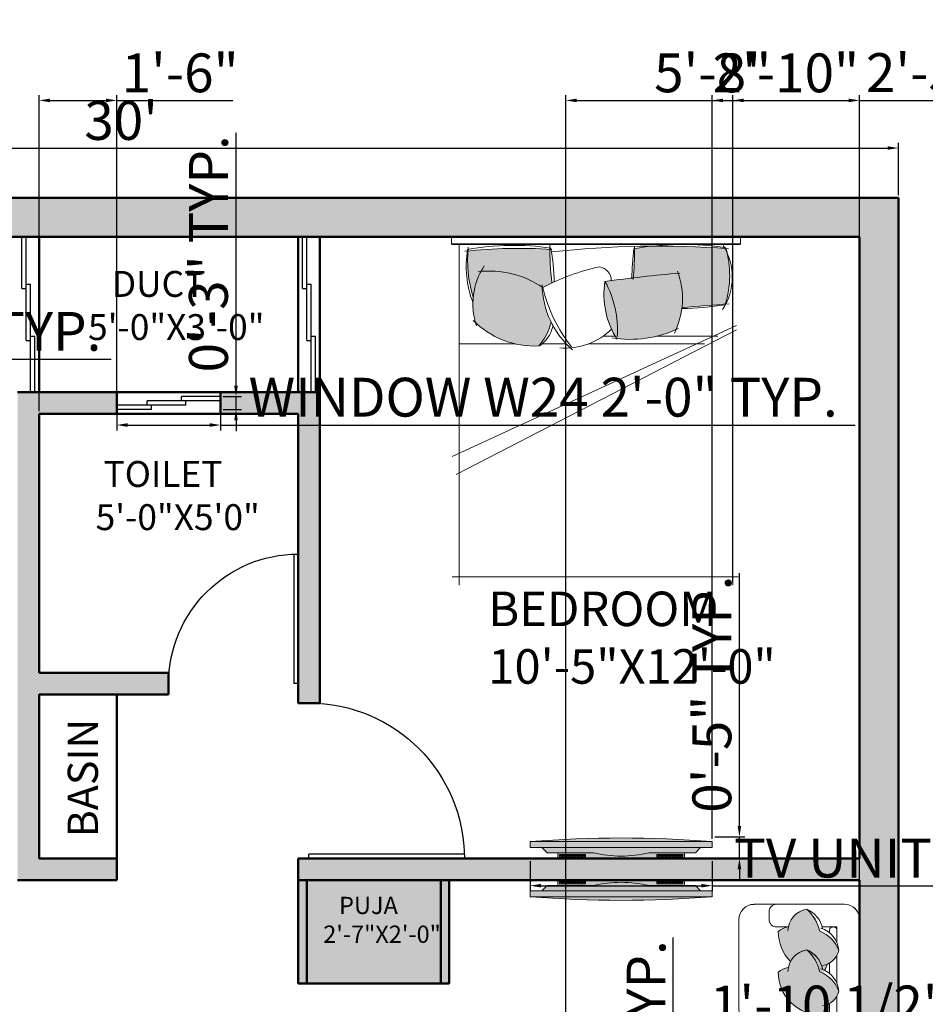
# Model space of a CAD drawing. Units: inches. Extents: x 3274 to 5176, y 1085 to 2172.
# Tile 8 of 16: x 3530 to 3740, y 1848 to 2076. Entities that reach past the tile are written whole.
import ezdxf

# ---------------------------------------------------------------- set-up
doc = ezdxf.new("R2010")
doc.units = ezdxf.units.IN
for name, color, linetype, lineweight in [('0.10', 252, 'Continuous', 9), ('A-ANNO-DIMS', 2, 'Continuous', 18), ('A-AREA-IDEN', 3, 'Continuous', 25), ('A-DOOR', 4, 'Continuous', 25), ('A-EQPM', 8, 'Continuous', 18), ('A-FLOR-PATT', 252, 'Continuous', 13), ('A-FURN', 8, 'Continuous', 18), ('A-GLAZ', 5, 'Continuous', 25), ('A-WALL', 7, 'Continuous', 50), ('A-WALL-PATT', 8, 'Continuous', 13), ('moveis', 254, 'Continuous', 5), ('parede', 7, 'Continuous', 30)]:
    doc.layers.add(name, color=color, linetype=linetype, lineweight=lineweight)
doc.styles.get("Standard").update_dxf_attribs({"font": 'arial.ttf'})
doc.dimstyles.new('ISO-25', dxfattribs={"dimtxt": 9, "dimasz": 2.5, "dimexe": 1.25, "dimexo": 0.625, "dimtad": 1, "dimdec": 1, "dimlunit": 3, "dimtxsty": 'Standard', "dimcen": 2.5, "dimclrd": 4, "dimclre": 4, "dimclrt": 1, "dimadec": 0, "dimazin": 0, "dimtfac": 1, "dimtdec": 1, "dimtmove": 0, "dimatfit": 3, "dimfxl": 1, "dimarcsym": 0})

# ---------------------------------------------------------------- blocks, each defined once
blk = doc.blocks.new('2')
for p, q in [((0, 30), (0, 0)), ((1, 30), (1, 0)), ((0, 0), (1, 0))]:
    blk.add_line(p, q)
blk.add_arc((0, 0), 30, 0, 90)
blk = doc.blocks.new('1')
for p, q in [((0, 36), (0, 0)), ((1, 36), (1, 0)), ((0, 0), (1, 0))]:
    blk.add_line(p, q)
blk.add_arc((0, 0), 36, 0, 90)
blk = doc.blocks.new('*D67')
at = {"layer": 'A-ANNO-DIMS', "color": 0, "lineweight": -2, "transparency": 16777216}
for p, q in [((3373.3, 2035.11), (3373.3, 2047.29)), ((3733.3, 2035.11), (3733.3, 2047.29)), ((3375.8, 2046.04), (3730.8, 2046.04))]:
    blk.add_line(p, q, dxfattribs=at)
at = {"layer": 'A-ANNO-DIMS', "color": 0, "transparency": 16777216}
for points in [[(3375.8, 2046.46), (3375.8, 2045.63), (3373.3, 2046.04)], [(3730.8, 2046.46), (3730.8, 2045.63), (3733.3, 2046.04)]]:
    blk.add_solid(points, dxfattribs=at)
at = {"layer": 'Defpoints', "color": 0, "transparency": 16777216}
for p in [(3733.3, 2046.04), (3373.3, 2034.48), (3733.3, 2034.48)]:
    blk.add_point(p, dxfattribs=at)
at = {"layer": 'A-ANNO-DIMS', "color": 0, "transparency": 16777216, "insert": (3553.3, 2051.27), "char_height": 9, "attachment_point": 5}
blk.add_mtext("30'", dxfattribs=at)
blk = doc.blocks.new('camita')
at = {"layer": '0.10'}
for p, q in [((-0.85, -0.045), (0.85, -0.045)), ((-0.805, -0.045), (-0.805, -2.0485)), ((0.805, -0.045), (0.805, -2.0485)), ((-0.8271, -0.521), (0.8464, -1.2932)), ((-0.8271, -0.5476), (0.8236, -1.3992)), ((-0.7161, -0.585), (-0.3554, -0.585)), ((-0.638, -0.63), (0.0434, -0.63)), ((-0.1136, -0.585), (-0.0485, -0.585)), ((0.1749, -0.63), (0.3179, -0.63)), ((0.4739, -0.63), (0.805, -0.63)), ((-0.8354, -2), (0.8464, -2))]:
    blk.add_line(p, q, dxfattribs=at)
blk.add_lwpolyline([(-0.85, -0.0405), (0.85, -0.0405), (0.85, 0), (-0.85, 0)], close=True, dxfattribs=at)
for centre, radius, start, end in [((-0.4574, -0.2364), 0.3443, 147.50996, 213.83359), ((-0.3639, -5.8457), 5.7909, 83.80731, 94.12107), ((-0.5104, -1.7232), 1.6781, 80.12554, 98.66187), ((-1.4396, -0.0609), 1.7117, 352.92911, 0.39592), ((0.4863, -1.6286), 1.5781, 80.16015, 98.05996), ((-0.1997, -0.2266), 0.5864, 163.92635, 197.14087), ((2.3534, -0.0532), 2.5803, 180.10628, 184.38541), ((-1.5443, -0.2452), 1.3333, 359.93941, 7.55329), ((1.5815, -0.2893), 1.3353, 170.38021, 178.99138), ((0.4524, -3.0675), 2.9996, 83.90257, 93.67595), ((0.0294, -0.1377), 0.7262, 342.58415, 6.00484), ((0.1326, -0.1696), 0.6307, 339.92303, 8.74334), ((0.3203, -0.3944), 0.4043, 341.45245, 33.45121), ((-0.0543, -0.3633), 0.4542, 159.30257, 206.50263), ((-1.3301, -9.6748), 9.4985, 82.27078, 84.93989), ((-0.007, -0.258), 0.0828, 100.01798, 179.73597), ((-0.2931, -1.4378), 1.2903, 61.97485, 77.84351), ((0.6265, -0.7518), 0.5508, 82.96906, 124.67388), ((0.4585, -0.5454), 0.5842, 151.04555, 184.14969), ((-0.5341, -0.3393), 0.4875, 327.26442, 9.0473), ((-0.1986, -0.2742), 0.5159, 310.73945, 359.05759), ((-0.5673, -0.0868), 0.9057, 321.69527, 346.46261), ((-1.8672, -14.986), 14.6323, 84.65974, 85.75157), ((-0.4598, 1.4861), 1.9092, 260.95299, 268.65169), ((0.5707, -0.4317), 0.3145, 192.93877, 221.96363), ((0.3612, -0.133), 0.5096, 267.25889, 315.29965), ((-0.2002, 0.064), 0.6673, 244.78094, 279.06058), ((0.179, -0.272), 0.3828, 224.52836, 275.22287), ((0.4384, -0.4834), 0.1898, 193.68485, 236.70352)]:
    blk.add_arc(centre, radius, start, end, dxfattribs=at)
blk = doc.blocks.new('SOFA 1')
at = {"transparency": 33554687}
h = blk.add_hatch(color=256, dxfattribs=at)
h.dxf.hatch_style = 1
h.paths.add_polyline_path([(3723.52, 1308.63, 0.147724), (3717.76, 1305.24, 0.310469), (3722.42, 1300.4), (3722.42, 1300.25, 0.156703), (3723.62, 1297.8, 0.425821), (3734.69, 1309.08, 0.121928), (3732.05, 1310.63, 0.233216), (3728.6, 1313.59, 0.213835)])
h = blk.add_hatch(color=256, dxfattribs=at)
h.dxf.hatch_style = 1
h.paths.add_polyline_path([(3769.65, 1307.6, 0.084911), (3767.15, 1309.12, 0.046133), (3766.46, 1311.13), (3759.18, 1311.13, 0.039409), (3758.92, 1310.24, 0.165523), (3756.31, 1309.02, 0.42585), (3767.59, 1297.95, 0.121928), (3769.15, 1300.58, 0.027403), (3769.65, 1300.83)])
h.paths.add_polyline_path([(3765.34, 1313.08), (3760.4, 1313.08, 0.097704), (3759.18, 1311.13), (3766.46, 1311.13, 0.04873)])
h.paths.add_polyline_path([(3763.76, 1314.88, 0.16488), (3760.4, 1313.08), (3765.34, 1313.08, 0.051917)])
h.paths.add_polyline_path([(3771.6, 1305.17, 0.090388), (3769.65, 1307.6), (3769.65, 1300.83, 0.136035), (3771.6, 1302.77)])
h = blk.add_hatch(color=256, dxfattribs=at)
h.dxf.hatch_style = 1
h.paths.add_polyline_path([(3769.16, 1235.96, 0.122267), (3767.6, 1238.61, 0.425972), (3756.32, 1227.54, 0.165563), (3758.93, 1226.32, 0.309481), (3763.76, 1221.69, 0.002677), (3763.83, 1221.72, 0.146094), (3767.16, 1227.43, 0.212433), (3772.1, 1232.48, 0.235342)])
h = blk.add_hatch(color=256, dxfattribs=at)
h.dxf.hatch_style = 1
h.paths.add_polyline_path([(3769.16, 1225.36, 0.122267), (3767.6, 1228.01, 0.425972), (3756.32, 1216.94, 0.165563), (3758.93, 1215.72, 0.309481), (3763.76, 1211.09, 0.002677), (3763.83, 1211.12, 0.146094), (3767.16, 1216.83, 0.212433), (3772.1, 1221.88, 0.235342)])
for p, q in [((3720.45, 1316.13), (3773.58, 1316.13)), ((3777.51, 1312.19), (3777.51, 1213.72))]:
    blk.add_line(p, q, dxfattribs=at)
for points in [[(3717.76, 1305.24, -0.147724), (3723.52, 1308.63, -0.213355), (3728.59, 1313.59, 0.213355), (3723.52, 1308.63, 0.147724), (3717.76, 1305.24, -0.249545), (3722.86, 1309.34, 0.249545), (3717.75, 1305.25, 0.356779), (3723.4, 1300.28, -0.356779), (3717.76, 1305.24)], [(3728.58, 1313.6, -0.306333), (3732.42, 1309.31, 0.306333), (3728.58, 1313.6, 0.306674), (3722.72, 1308.89, -0.306674), (3728.58, 1313.6)], [(3763.76, 1314.88, -0.147724), (3767.15, 1309.12, -0.213355), (3772.1, 1304.05, 0.213355), (3767.15, 1309.12, 0.147724), (3763.76, 1314.88, -0.249545), (3767.86, 1309.77, 0.249545), (3763.77, 1314.89, 0.356779), (3758.8, 1309.23, -0.356779), (3763.76, 1314.88)], [(3734.69, 1309.08, -0.425972), (3723.62, 1297.8, -0.165552), (3722.4, 1300.4, 0.165552), (3723.62, 1297.79, 0.425972), (3734.69, 1309.07, 0.121514), (3732.07, 1310.63, -0.121514), (3734.69, 1309.08)], [(3767.6, 1297.95, -0.425972), (3756.31, 1309.01, -0.165552), (3758.92, 1310.24, 0.165552), (3756.31, 1309.02, 0.425972), (3767.59, 1297.95, 0.121514), (3769.14, 1300.57, -0.121514), (3767.6, 1297.95)], [(3772.11, 1304.06, -0.306333), (3767.83, 1300.22, 0.306333), (3772.11, 1304.06, 0.306674), (3767.4, 1309.91, -0.306674), (3772.11, 1304.06)], [(3770.44, 1286.63, -0.414214), (3769.66, 1287.4, 0.414214), (3770.44, 1286.63, 0.414214), (3769.66, 1285.83, -0.414214), (3770.44, 1286.63)], [(3748.01, 1262.99, -0.414214), (3746.05, 1264.95, 0.414214), (3748.01, 1262.97, 0.414213), (3746.05, 1261.01, -0.414213), (3748.01, 1262.99)], [(3770.44, 1262.99, -0.414214), (3769.66, 1263.77, 0.414214), (3770.44, 1262.99, 0.414214), (3769.66, 1262.19, -0.414214), (3770.44, 1262.99)], [(3770.83, 1262.97, -0.414214), (3771.61, 1262.19, 0.414214), (3770.83, 1262.99, 0.414214), (3771.61, 1263.77, -0.414214), (3770.83, 1262.97)], [(3748.01, 1239.35, -0.414214), (3746.05, 1241.31, 0.414214), (3748.01, 1239.33, 0.414213), (3746.05, 1237.37, -0.414213), (3748.01, 1239.35)], [(3767.7, 1239.33, -0.414214), (3769.66, 1237.37, 0.414214), (3767.7, 1239.35, 0.414214), (3769.66, 1241.31, -0.414214), (3767.7, 1239.33)], [(3756.32, 1227.54, -0.425972), (3767.6, 1238.61, -0.121514), (3769.16, 1235.98, 0.121514), (3767.6, 1238.61, 0.425972), (3756.32, 1227.54, 0.165552), (3758.93, 1226.32, -0.165552), (3756.32, 1227.54)], [(3770.44, 1239.35, -0.414214), (3769.66, 1240.13, 0.414214), (3770.44, 1239.33, 0.414214), (3769.66, 1238.55, -0.414214), (3770.44, 1239.35)], [(3770.83, 1239.33, -0.414214), (3771.61, 1238.55, 0.414214), (3770.83, 1239.35, 0.414214), (3771.61, 1240.13, -0.414214), (3770.83, 1239.33)], [(3772.1, 1232.5, -0.306674), (3767.41, 1226.64, 0.306674), (3772.1, 1232.5, 0.306333), (3767.84, 1236.34, -0.306333), (3772.1, 1232.5)], [(3763.78, 1221.67, 0.249545), (3767.87, 1226.78, -0.249545), (3763.76, 1221.69, -0.356779), (3758.81, 1227.32, 0.356779), (3763.77, 1221.68, 0.147724), (3767.16, 1227.43, 0.213355), (3772.11, 1232.51, -0.213355), (3767.16, 1227.43, -0.147724), (3763.78, 1221.67)], [(3756.32, 1216.94, -0.200233), (3759.49, 1224.76, 0.200233), (3756.32, 1216.94, 0.165552), (3758.93, 1215.72, -0.165552), (3756.32, 1216.94)], [(3772.1, 1221.9, -0.306674), (3767.41, 1216.04, 0.306674), (3772.1, 1221.9, -0.213355), (3767.16, 1216.83, -0.147724), (3763.77, 1211.08, 0.147724), (3767.15, 1216.83, 0.213355), (3772.1, 1221.9)], [(3763.76, 1211.09, -0.356779), (3758.81, 1216.72, 0.356779), (3763.76, 1211.09, 0.249545), (3767.87, 1216.18, -0.249545), (3763.76, 1211.09)]]:
    blk.add_lwpolyline(points, format="xyb", dxfattribs=at)
for points in [[(3716.51, 1312.2), (3716.51, 1291.44)], [(3722.42, 1313.08), (3722.42, 1309.23), (3722.42, 1313.08), (3726.57, 1313.08)], [(3723.21, 1311.13), (3723.93, 1311.13)], [(3729.85, 1313.08), (3745.25, 1313.08)], [(3731.82, 1311.13), (3745.25, 1311.13)], [(3746.01, 1312.3), (3746.01, 1288.55)], [(3746.01, 1310.97), (3746.01, 1311.36)], [(3768.11, 1313.08), (3746.78, 1313.08)], [(3768.87, 1311.13), (3746.78, 1311.13)], [(3771.6, 1313.08), (3767.75, 1313.08), (3771.6, 1313.08), (3771.6, 1308.93)], [(3769.66, 1287.39), (3769.65, 1312.3)], [(3771.6, 1313.08), (3771.61, 1233.74)], [(3746.01, 1288.54), (3746.01, 1308.23)], [(3769.65, 1309.43), (3769.65, 1308.71)], [(3722.42, 1300.39), (3722.42, 1297.33)], [(3720.45, 1295.38), (3718.48, 1295.38)], [(3720.45, 1287.5), (3744.09, 1287.5)], [(3747.99, 1286.6), (3767.69, 1286.6)], [(3769.66, 1263.75), (3769.66, 1285.81)], [(3746.02, 1284.63), (3746.02, 1264.94)], [(3769.66, 1277.18), (3769.66, 1263.75)], [(3747.99, 1262.97), (3767.69, 1262.97)], [(3769.66, 1240.12), (3769.66, 1262.18)], [(3770.43, 1262.97), (3770.82, 1262.97)], [(3746.02, 1260.99), (3746.02, 1241.3)], [(3747.99, 1239.33), (3767.69, 1239.33)], [(3770.43, 1239.33), (3770.82, 1239.33)], [(3746.02, 1237.36), (3746.02, 1213.74)], [(3769.66, 1235.71), (3769.66, 1238.54)], [(3771.61, 1223.14), (3771.61, 1230.47)], [(3769.66, 1225.11), (3769.66, 1227.82)], [(3767.76, 1215.72), (3771.61, 1215.72), (3771.61, 1219.84), (3771.61, 1215.72)], [(3755.86, 1215.72), (3758.92, 1215.72)], [(3769.66, 1216.5), (3769.66, 1217.22)], [(3753.91, 1211.77), (3753.91, 1213.74)], [(3749.97, 1209.8), (3773.58, 1209.8)]]:
    blk.add_lwpolyline(points, close=True, dxfattribs=at)
for points in [[(3722.42, 1311.91, 0.414214), (3723.2, 1311.13, -0.414214)], [(3770.43, 1313.08, 0.414214), (3769.65, 1312.3, -0.414214)], [(3771.6, 1312.3, 0.414214), (3770.82, 1313.08, -0.414214)], [(3716.51, 1297.34, 0.414214), (3718.47, 1295.38, -0.414214)], [(3720.44, 1295.38, 0.414214), (3722.4, 1297.34, -0.414214)], [(3716.51, 1291.45, 0.414212), (3720.44, 1287.52, -0.414212)], [(3746.03, 1288.56, 0.414214), (3747.99, 1286.6, 0.414213), (3746.03, 1284.64, -0.414213), (3747.99, 1286.6, -0.414214)], [(3769.66, 1284.64, 0.414214), (3767.7, 1286.6, 0.414214), (3769.66, 1288.56, -0.414214), (3767.7, 1286.6, -0.414214)], [(3769.66, 1261.01, 0.414214), (3767.7, 1262.97, 0.414214), (3769.66, 1264.93, -0.414214), (3767.7, 1262.97, -0.414214)], [(3769.16, 1225.36, 0.071861), (3768.39, 1227.01, -0.071861)], [(3772.13, 1221.9, 0.306333), (3767.84, 1225.74, -0.306333)], [(3755.87, 1215.72, 0.414214), (3753.91, 1213.76, -0.414214)], [(3769.66, 1216.52, 0.414214), (3770.44, 1215.74, -0.414214)], [(3770.83, 1215.74, 0.414214), (3771.61, 1216.52, -0.414214)], [(3746.05, 1213.76, 0.414212), (3749.98, 1209.82, -0.414212)], [(3755.87, 1209.8, -0.414214), (3753.91, 1211.76, 0.414214)]]:
    blk.add_lwpolyline(points, format="xyb", close=True, dxfattribs=at)
for centre, radius, start, end in [((3720.44, 1312.2), 3.93, 90.0002, 179.9998), ((3720.44, 1312.19), 3.94, 89.9158, 179.9154), ((3773.58, 1312.2), 3.93, 0.0002, 89.9998), ((3773.57, 1312.19), 3.94, 359.9158, 89.9154), ((3744.09, 1309.21), 1.92, 358.766, 90.5111), ((3745.22, 1312.29), 0.789, 0.8425, 90.8425), ((3745.24, 1311.91), 0.777, 270, 0), ((3745.24, 1311.91), 0.777, 270, 0), ((3746.8, 1312.29), 0.789, 89.1575, 179.1575), ((3746.79, 1311.91), 0.777, 180, 270), ((3746.79, 1311.91), 0.777, 180, 270), ((3747.93, 1309.21), 1.92, 89.4889, 181.234), ((3768.87, 1312.3), 0.777, 360, 90), ((3768.87, 1311.91), 0.777, 270, 0), ((3744.08, 1289.48), 1.96, 270, 360), ((3744.08, 1289.48), 1.96, 270, 360), ((3773.58, 1213.73), 3.93, 270.0002, 359.9998), ((3773.59, 1213.73), 3.93, 269.9156, 359.9152)]:
    blk.add_arc(centre, radius, start, end, dxfattribs=at)
blk = doc.blocks.new('PLASMA 2')
at = {"layer": 'moveis', "ltscale": 0.08}
h = blk.add_hatch(dxfattribs=at)
h.set_pattern_fill('_USER,_O', color=256, scale=0.008, double=1, pattern_type=0)
h.set_pattern_definition([(360, (-4.134502, -6.848382), (0, 0.008), []), (90, (-4.134502, -6.848382), (-0.008, 0), [])])
h.paths.add_polyline_path([(-0.2099, -0.0965), (-0.3623, -0.0965), (-0.3623, -0.1111), (-0.2099, -0.1111)])
h = blk.add_hatch(dxfattribs=at)
h.set_pattern_fill('_USER,_O', color=256, scale=0.008, double=1, pattern_type=0)
h.set_pattern_definition([(180, (4.134502, -6.848382), (0, 0.008), []), (90, (4.134502, -6.848382), (0.008, 0), [])])
h.paths.add_polyline_path([(0.2099, -0.0965), (0.3623, -0.0965), (0.3623, -0.1111), (0.2099, -0.1111)])
at = {"layer": 'parede', "ltscale": 0.08}
h = blk.add_hatch(color=256, dxfattribs=at)
h.dxf.hatch_style = 1
h.set_gradient(color1=(131, 136, 145), one_color=1, tint=1, name='CURVED')
h.paths.add_polyline_path([(-0.535, -0.0215), (0.535, -0.0215, 0.040195)])
h = blk.add_hatch(color=256, dxfattribs=at)
h.dxf.hatch_style = 1
h.set_gradient(color1=(131, 136, 145), color2=(0, 0, 0), one_color=1, name='CURVED')
h.paths.add_polyline_path([(0.535, -0.0215), (-0.535, -0.0215), (-0.535, -0.0553), (0.535, -0.0553)])
h = blk.add_hatch(color=256, dxfattribs=at)
h.dxf.hatch_style = 1
h.set_gradient(color1=(131, 136, 145), one_color=1, tint=1, name='CYLINDER')
h.paths.add_polyline_path([(0.4673, -0.0553), (-0.4673, -0.0553), (-0.4363, -0.0876), (-0.1636, -0.0876, 0.114423), (0.1636, -0.0876), (0.4363, -0.0876)])
h = blk.add_hatch(color=256, dxfattribs=at)
h.dxf.hatch_style = 1
h.set_gradient(color1=(131, 136, 145), color2=(0, 0, 0), one_color=1, name='CURVED')
h.paths.add_polyline_path([(0.3724, -0.0876), (0.1636, -0.0876, -0.114423), (-0.1636, -0.0876), (-0.3724, -0.0876), (-0.3724, -0.12), (0.3724, -0.12)])
h.paths.add_polyline_path([(-0.2099, -0.1111), (-0.3623, -0.1111), (-0.3623, -0.0965), (-0.2099, -0.0965)], flags=16)
h.paths.add_polyline_path([(0.2099, -0.1111), (0.2099, -0.0965), (0.3623, -0.0965), (0.3623, -0.1111)], flags=16)
at = {"layer": 'moveis', "ltscale": 0.08}
for p, q in [((-0.535, -0.0215), (-0.535, -0.0553)), ((-0.535, -0.0215), (0.535, -0.0215)), ((0.535, -0.0553), (-0.535, -0.0553)), ((-0.4673, -0.0553), (-0.4363, -0.0876)), ((0.4673, -0.0553), (0.4363, -0.0876)), ((0.535, -0.0553), (0.535, -0.0215)), ((-0.4363, -0.0876), (-0.1636, -0.0876)), ((-0.3724, -0.0876), (-0.3724, -0.12)), ((0.1636, -0.0876), (0.4363, -0.0876)), ((0.3724, -0.0876), (0.3724, -0.12)), ((-0.3724, -0.12), (0.3724, -0.12))]:
    blk.add_line(p, q, dxfattribs=at)
for points in [[(-0.3623, -0.0965), (-0.2099, -0.0965), (-0.2099, -0.1111), (-0.3623, -0.1111)], [(0.3623, -0.0965), (0.2099, -0.0965), (0.2099, -0.1111), (0.3623, -0.1111)]]:
    blk.add_lwpolyline(points, close=True, dxfattribs=at)
for centre, radius, start, end in [((0, -6.6658), 6.6658, 85.39647, 94.60353), ((0, 0.6178), 0.7242, 256.94486, 283.05514)]:
    blk.add_arc(centre, radius, start, end, dxfattribs=at)
blk = doc.blocks.new('WIN-24')
for p, q in [((4551.19, 1486.35), (4551.19, 1487.35)), ((4560.19, 1487.35), (4551.19, 1487.35)), ((4552.19, 1485.35), (4536.19, 1485.35)), ((4560.19, 1486.35), (4543.19, 1486.35)), ((4543.19, 1485.35), (4543.19, 1486.35)), ((4544.19, 1484.35), (4544.19, 1485.35)), ((4552.19, 1485.35), (4552.19, 1486.35)), ((4544.19, 1484.35), (4536.19, 1484.35))]:
    blk.add_line(p, q)
blk = doc.blocks.new('WIN-36')
for p, q in [((4514.19, 1512.35), (4514.19, 1524.35)), ((4515.19, 1500.35), (4515.19, 1524.35)), ((4514.19, 1512.35), (4515.19, 1512.35)), ((4515.19, 1513.35), (4516.19, 1513.35)), ((4516.19, 1488.35), (4516.19, 1513.35)), ((4516.19, 1501.35), (4517.19, 1501.35)), ((4517.19, 1488.35), (4517.19, 1501.35)), ((4515.19, 1500.35), (4516.19, 1500.35))]:
    blk.add_line(p, q)
blk = doc.blocks.new('*D126')
at = {"layer": 'A-ANNO-DIMS', "color": 4, "lineweight": -2, "transparency": 16777216}
for p, q in [((3552.3, 1984.86), (3552.3, 1980.63)), ((3576.3, 1984.86), (3576.3, 1980.63)), ((3554.8, 1981.88), (3573.8, 1981.88)), ((3576.3, 1981.88), (3723.28, 1981.88))]:
    blk.add_line(p, q, dxfattribs=at)
at = {"layer": 'A-ANNO-DIMS', "color": 4, "transparency": 16777216}
for points in [[(3554.8, 1982.3), (3554.8, 1981.47), (3552.3, 1981.88)], [(3573.8, 1982.3), (3573.8, 1981.47), (3576.3, 1981.88)]]:
    blk.add_solid(points, dxfattribs=at)
at = {"layer": 'Defpoints', "color": 0, "transparency": 16777216}
for p in [(3552.3, 1985.48), (3576.3, 1985.48), (3576.3, 1981.88)]:
    blk.add_point(p, dxfattribs=at)
at = {"layer": 'A-ANNO-DIMS', "color": 1, "transparency": 16777216, "insert": (3651.04, 1987.16), "char_height": 9, "attachment_point": 5}
blk.add_mtext('WINDOW W24 2\'-0" TYP.', dxfattribs=at)
blk = doc.blocks.new('*D127')
at = {"layer": 'A-ANNO-DIMS', "color": 4, "lineweight": -2, "transparency": 16777216}
for p, q in [((3579.9, 1990.98), (3579.9, 2049.59)), ((3576.93, 1988.48), (3581.15, 1988.48)), ((3579.9, 1985.48), (3579.9, 1988.48)), ((3576.93, 1985.48), (3581.15, 1985.48)), ((3579.9, 1982.98), (3579.9, 1980.48))]:
    blk.add_line(p, q, dxfattribs=at)
at = {"layer": 'A-ANNO-DIMS', "color": 4, "transparency": 16777216}
for points in [[(3579.48, 1990.98), (3580.32, 1990.98), (3579.9, 1988.48)], [(3579.48, 1982.98), (3580.32, 1982.98), (3579.9, 1985.48)]]:
    blk.add_solid(points, dxfattribs=at)
at = {"layer": 'Defpoints', "color": 0, "transparency": 16777216}
for p in [(3576.3, 1988.48), (3579.9, 1988.48), (3576.3, 1985.48)]:
    blk.add_point(p, dxfattribs=at)
at = {"layer": 'A-ANNO-DIMS', "color": 1, "transparency": 16777216, "insert": (3574.68, 2021.54), "char_height": 9, "attachment_point": 5, "rotation": 90}
blk.add_mtext('0\'-3" TYP.', dxfattribs=at)
blk = doc.blocks.new('*D130')
at = {"layer": 'A-ANNO-DIMS', "color": 4, "lineweight": -2, "transparency": 16777216}
for p, q in [((3648.04, 1880.86), (3648.04, 1873.91)), ((3690.17, 1880.86), (3690.17, 1873.91)), ((3650.54, 1875.16), (3687.67, 1875.16)), ((3690.17, 1875.16), (3801.39, 1875.16))]:
    blk.add_line(p, q, dxfattribs=at)
at = {"layer": 'A-ANNO-DIMS', "color": 4, "transparency": 16777216}
for points in [[(3650.54, 1875.58), (3650.54, 1874.75), (3648.04, 1875.16)], [(3687.67, 1875.58), (3687.67, 1874.75), (3690.17, 1875.16)]]:
    blk.add_solid(points, dxfattribs=at)
at = {"layer": 'Defpoints', "color": 0, "transparency": 16777216}
for p in [(3648.04, 1881.48), (3690.17, 1881.48), (3690.17, 1875.16)]:
    blk.add_point(p, dxfattribs=at)
at = {"layer": 'A-ANNO-DIMS', "color": 1, "transparency": 16777216, "insert": (3747.03, 1880.39), "char_height": 9, "attachment_point": 5}
blk.add_mtext('TV UNIT 3\'-6" TYP.', dxfattribs=at)
blk = doc.blocks.new('*D131')
at = {"layer": 'A-ANNO-DIMS', "color": 4, "lineweight": -2, "transparency": 16777216}
for p, q in [((3696.49, 1888.99), (3696.49, 1947.6)), ((3690.79, 1886.49), (3697.74, 1886.49)), ((3696.49, 1881.48), (3696.49, 1886.49)), ((3690.79, 1881.48), (3697.74, 1881.48)), ((3696.49, 1878.98), (3696.49, 1876.48))]:
    blk.add_line(p, q, dxfattribs=at)
at = {"layer": 'A-ANNO-DIMS', "color": 4, "transparency": 16777216}
for points in [[(3696.07, 1888.99), (3696.9, 1888.99), (3696.49, 1886.49)], [(3696.07, 1878.98), (3696.9, 1878.98), (3696.49, 1881.48)]]:
    blk.add_solid(points, dxfattribs=at)
at = {"layer": 'Defpoints', "color": 0, "transparency": 16777216}
for p in [(3690.17, 1886.49), (3696.49, 1886.49), (3690.17, 1881.48)]:
    blk.add_point(p, dxfattribs=at)
at = {"layer": 'A-ANNO-DIMS', "color": 1, "transparency": 16777216, "insert": (3691.27, 1919.54), "char_height": 9, "attachment_point": 5, "rotation": 90}
blk.add_mtext('0\'-5" TYP.', dxfattribs=at)
blk = doc.blocks.new('*D139')
at = {"layer": 'A-ANNO-DIMS', "color": 4, "lineweight": -2, "transparency": 16777216}
for p, q in [((3664.71, 1838.01), (3664.71, 1842.31)), ((3667.21, 1841.06), (3684.52, 1841.06)), ((3687.02, 1838.01), (3687.02, 1842.31)), ((3687.02, 1841.06), (3772.75, 1841.06))]:
    blk.add_line(p, q, dxfattribs=at)
at = {"layer": 'A-ANNO-DIMS', "color": 4, "transparency": 16777216}
for points in [[(3667.21, 1841.48), (3667.21, 1840.65), (3664.71, 1841.06)], [(3684.52, 1841.48), (3684.52, 1840.65), (3687.02, 1841.06)]]:
    blk.add_solid(points, dxfattribs=at)
at = {"layer": 'Defpoints', "color": 0, "transparency": 16777216}
for p in [(3687.02, 1841.06), (3664.71, 1837.38), (3687.02, 1837.38)]:
    blk.add_point(p, dxfattribs=at)
at = {"layer": 'A-ANNO-DIMS', "color": 1, "transparency": 16777216, "insert": (3731.13, 1846.34), "char_height": 9, "attachment_point": 5}
blk.add_mtext('1\'-10 1/2" TYP.', dxfattribs=at)
blk = doc.blocks.new('*D141')
at = {"layer": 'A-ANNO-DIMS', "color": 4, "lineweight": -2, "transparency": 16777216}
for p, q in [((3681.18, 1804.42), (3681.18, 1863.19)), ((3670.79, 1804.42), (3682.43, 1804.42)), ((3681.18, 1778.97), (3681.18, 1801.92)), ((3670.79, 1776.47), (3682.43, 1776.47))]:
    blk.add_line(p, q, dxfattribs=at)
at = {"layer": 'A-ANNO-DIMS', "color": 4, "transparency": 16777216}
for points in [[(3680.76, 1801.92), (3681.59, 1801.92), (3681.18, 1804.42)], [(3680.76, 1778.97), (3681.59, 1778.97), (3681.18, 1776.47)]]:
    blk.add_solid(points, dxfattribs=at)
at = {"layer": 'Defpoints', "color": 0, "transparency": 16777216}
for p in [(3670.16, 1804.42), (3681.18, 1804.42), (3670.16, 1776.47)]:
    blk.add_point(p, dxfattribs=at)
at = {"layer": 'A-ANNO-DIMS', "color": 1, "transparency": 16777216, "insert": (3676.03, 1835.06), "char_height": 9, "attachment_point": 5, "rotation": 90}
blk.add_mtext('2\'-4" TYP.', dxfattribs=at)
blk = doc.blocks.new('*D144')
at = {"layer": 'A-ANNO-DIMS', "color": 4, "lineweight": -2, "transparency": 16777216}
for p, q in [((3382.3, 2005.96), (3382.3, 1995.89)), ((3445.29, 2005.96), (3445.29, 1995.89)), ((3384.8, 1997.14), (3442.79, 1997.14)), ((3445.29, 1997.14), (3551.01, 1997.14))]:
    blk.add_line(p, q, dxfattribs=at)
at = {"layer": 'A-ANNO-DIMS', "color": 4, "transparency": 16777216}
for points in [[(3384.8, 1997.55), (3384.8, 1996.72), (3382.3, 1997.14)], [(3442.79, 1997.55), (3442.79, 1996.72), (3445.29, 1997.14)]]:
    blk.add_solid(points, dxfattribs=at)
at = {"layer": 'Defpoints', "color": 0, "transparency": 16777216}
for p in [(3382.3, 2006.59), (3445.29, 2006.59), (3445.29, 1997.14)]:
    blk.add_point(p, dxfattribs=at)
at = {"layer": 'A-ANNO-DIMS', "color": 1, "transparency": 16777216, "insert": (3499.4, 2002.42), "char_height": 9, "attachment_point": 5}
blk.add_mtext('BENCH 5\'-3" TYP.', dxfattribs=at)
blk = doc.blocks.new('*D174')
at = {"layer": 'A-ANNO-DIMS', "color": 4, "lineweight": -2, "transparency": 16777216}
for p, q in [((3656.3, 1777.11), (3656.3, 2058.33)), ((3724.3, 1777.11), (3724.3, 2058.33)), ((3658.8, 2057.08), (3721.8, 2057.08))]:
    blk.add_line(p, q, dxfattribs=at)
at = {"layer": 'A-ANNO-DIMS', "color": 4, "transparency": 16777216}
for points in [[(3658.8, 2057.5), (3658.8, 2056.67), (3656.3, 2057.08)], [(3721.8, 2057.5), (3721.8, 2056.67), (3724.3, 2057.08)]]:
    blk.add_solid(points, dxfattribs=at)
at = {"layer": 'Defpoints', "color": 0, "transparency": 16777216}
for p in [(3724.3, 2057.08), (3656.3, 1776.48), (3724.3, 1776.48)]:
    blk.add_point(p, dxfattribs=at)
at = {"layer": 'A-ANNO-DIMS', "color": 1, "transparency": 16777216, "insert": (3690.3, 2062.3), "char_height": 9, "attachment_point": 5}
blk.add_mtext('5\'-8"', dxfattribs=at)
blk = doc.blocks.new('*D175')
at = {"layer": 'A-ANNO-DIMS', "color": 4, "lineweight": -2, "transparency": 16777216}
for p, q in [((3534.3, 1985.11), (3534.3, 2058.33)), ((3552.3, 1985.11), (3552.3, 2058.33)), ((3536.8, 2057.08), (3549.8, 2057.08)), ((3552.3, 2057.08), (3579.13, 2057.08))]:
    blk.add_line(p, q, dxfattribs=at)
at = {"layer": 'A-ANNO-DIMS', "color": 4, "transparency": 16777216}
for points in [[(3536.8, 2057.5), (3536.8, 2056.67), (3534.3, 2057.08)], [(3549.8, 2057.5), (3549.8, 2056.67), (3552.3, 2057.08)]]:
    blk.add_solid(points, dxfattribs=at)
at = {"layer": 'Defpoints', "color": 0, "transparency": 16777216}
for p in [(3552.3, 2057.08), (3534.3, 1984.48), (3552.3, 1984.48)]:
    blk.add_point(p, dxfattribs=at)
at = {"layer": 'A-ANNO-DIMS', "color": 1, "transparency": 16777216, "insert": (3566.96, 2062.3), "char_height": 9, "attachment_point": 5}
blk.add_mtext('1\'-6"', dxfattribs=at)
blk = doc.blocks.new('*D177')
at = {"layer": 'A-ANNO-DIMS', "color": 4, "lineweight": -2, "transparency": 16777216}
for p, q in [((3694.98, 1945.45), (3694.98, 2058.33)), ((3724.3, 1882.11), (3724.3, 2058.33)), ((3697.48, 2057.08), (3721.8, 2057.08)), ((3724.3, 2057.08), (3773.1, 2057.08))]:
    blk.add_line(p, q, dxfattribs=at)
at = {"layer": 'A-ANNO-DIMS', "color": 4, "transparency": 16777216}
for points in [[(3697.48, 2057.5), (3697.48, 2056.67), (3694.98, 2057.08)], [(3721.8, 2057.5), (3721.8, 2056.67), (3724.3, 2057.08)]]:
    blk.add_solid(points, dxfattribs=at)
at = {"layer": 'Defpoints', "color": 0, "transparency": 16777216}
for p in [(3724.3, 2057.08), (3694.98, 1944.83), (3724.3, 1881.48)]:
    blk.add_point(p, dxfattribs=at)
at = {"layer": 'A-ANNO-DIMS', "color": 1, "transparency": 16777216, "insert": (3749.95, 2062.36), "char_height": 9, "attachment_point": 5}
blk.add_mtext('2\'-5 1/2"', dxfattribs=at)
blk = doc.blocks.new('*D179')
at = {"layer": 'A-ANNO-DIMS', "color": 4, "lineweight": -2, "transparency": 16777216}
for p, q in [((3690.17, 1885.99), (3690.17, 2058.33)), ((3724.3, 1882.11), (3724.3, 2058.33)), ((3692.67, 2057.08), (3721.8, 2057.08))]:
    blk.add_line(p, q, dxfattribs=at)
at = {"layer": 'A-ANNO-DIMS', "color": 4, "transparency": 16777216}
for points in [[(3692.67, 2057.5), (3692.67, 2056.67), (3690.17, 2057.08)], [(3721.8, 2057.5), (3721.8, 2056.67), (3724.3, 2057.08)]]:
    blk.add_solid(points, dxfattribs=at)
at = {"layer": 'Defpoints', "color": 0, "transparency": 16777216}
for p in [(3724.3, 2057.08), (3690.17, 1885.36), (3724.3, 1881.48)]:
    blk.add_point(p, dxfattribs=at)
at = {"layer": 'A-ANNO-DIMS', "color": 1, "transparency": 16777216, "insert": (3707.24, 2062.3), "char_height": 9, "attachment_point": 5}
blk.add_mtext('2\'-10"', dxfattribs=at)

msp = doc.modelspace()

# ---------------------------------------------------------------- hatches: boundary and pattern name
at = {"layer": 'A-FLOR-PATT'}
h = msp.add_hatch(color=256, dxfattribs=at)
h.dxf.hatch_style = 1
h.paths.add_polyline_path([(3693.63, 2021.8, 0.020657), (3693.12, 2022.8, 0.01851), (3676.25, 2023.32, 0.015442), (3672.21, 2022.76, -0.016701), (3671.94, 2015.98, -0.006967), (3682.31, 2017.05, -0.113891), (3683.18, 2009.06, -0.004387), (3693.25, 2009.91, 0.131047)])
h.paths.add_polyline_path([(3682.31, 2017.05, 0.006967), (3671.94, 2015.98, 0.00444), (3665.35, 2015.14, 0.181694), (3668.06, 2001.91, 0.134508), (3681.79, 2003.97, 0.189536)])
h = msp.add_hatch(color=256, dxfattribs=at)
h.dxf.hatch_style = 1
h.paths.add_polyline_path([(3652.57, 2022.6, 0.040212), (3633.61, 2022.21, 0.094792), (3634.83, 2011.54, -0.098488), (3636.64, 2017.48, -0.175864), (3650.95, 2013.72, -0.011742), (3653.08, 2014.79, -0.029051)])
h.paths.add_polyline_path([(3650.81, 2013.81, 0.173835), (3636.64, 2017.48, 0.194952), (3635.36, 2005.59, 0.202559), (3650.02, 2000.2, 0.127326), (3652.88, 2005.71, -0.104045)])
h = msp.add_hatch(color=256, dxfattribs=at)
h.dxf.hatch_style = 1
h.paths.add_polyline_path([(3629.3, 1876.48), (3627.3, 1876.48), (3627.3, 1852.48), (3629.3, 1852.48)])
h.paths.add_polyline_path([(3596.3, 1876.48), (3594.3, 1876.48), (3594.3, 1852.48), (3596.3, 1852.48)])
h = msp.add_hatch(color=256, dxfattribs=at)
h.dxf.hatch_style = 1
h.paths.add_polyline_path([(3627.3, 1876.48), (3596.3, 1876.48), (3596.3, 1852.48), (3627.3, 1852.48)])
h.paths.add_polyline_path([(3598.94, 1859.73), (3626.92, 1859.73), (3626.92, 1874.65), (3598.94, 1874.65)], flags=24)
at = {"layer": 'A-WALL-PATT'}
h = msp.add_hatch(color=256, dxfattribs=at)
h.dxf.hatch_style = 1
h.paths.add_polyline_path([(3733.3, 2034.48), (3373.3, 2034.48), (3373.3, 1674.48), (3406.3, 1674.48), (3406.3, 1683.48), (3382.3, 1683.48), (3382.3, 1767.48), (3442.3, 1767.48), (3442.3, 1772.48), (3382.3, 1772.48), (3382.3, 1876.48), (3442.3, 1876.48), (3442.3, 1881.48), (3382.3, 1881.48), (3382.3, 2025.48), (3724.3, 2025.48), (3724.3, 1881.48), (3594.3, 1881.48), (3594.3, 1876.48), (3724.3, 1876.48), (3724.3, 1776.48), (3656.3, 1776.48), (3656.3, 1767.48), (3724.3, 1767.48), (3724.3, 1683.48), (3682.3, 1683.48), (3682.3, 1674.48), (3733.3, 1674.48)])
h.paths.add_polyline_path([(3477.3, 1876.48), (3493.3, 1876.48), (3493.3, 1881.48), (3472.3, 1881.48), (3472.3, 1820.48), (3417.3, 1820.48), (3417.3, 1840.48), (3412.3, 1840.48), (3412.3, 1815.48), (3472.3, 1815.48), (3472.3, 1767.48), (3493.3, 1767.48), (3493.3, 1772.48), (3477.3, 1772.48)], flags=17)
h.paths.add_polyline_path([(3534.3, 1984.48), (3552.3, 1984.48), (3552.3, 1989.48), (3529.3, 1989.48), (3529.3, 1876.48), (3552.3, 1876.48), (3552.3, 1881.48), (3534.3, 1881.48), (3534.3, 1919.48), (3564.3, 1919.48), (3564.3, 1924.48), (3534.3, 1924.48)], flags=17)
h.paths.add_polyline_path([(3599.3, 1989.48), (3576.3, 1989.48), (3576.3, 1984.48), (3594.3, 1984.48), (3594.3, 1917.48), (3599.3, 1917.48)], flags=17)
h.paths.add_polyline_path([(3534.3, 1767.48), (3539.3, 1767.48), (3539.3, 1776.48), (3529.3, 1776.48), (3529.3, 1683.48), (3478.3, 1683.48), (3478.3, 1674.48), (3534.3, 1674.48)], flags=17)
h.paths.add_polyline_path([(3596.3, 1776.48), (3587.3, 1776.48), (3587.3, 1771.98), (3587.3, 1767.48), (3596.3, 1767.48)], flags=17)
h.paths.add_polyline_path([(3610.3, 1683.48), (3594.3, 1683.48), (3594.3, 1674.48), (3610.3, 1674.48)], flags=17)
h.paths.add_polyline_path([(3589.35, 1817.42), (3663.55, 1817.42), (3663.55, 1847.27), (3589.35, 1847.27)], flags=25)
h.paths.add_polyline_path([(3545.54, 1954.13), (3584.72, 1954.13), (3584.72, 1976.52), (3545.54, 1976.52)], flags=25)
h.paths.add_polyline_path([(3635.11, 1944.89), (3703.51, 1944.89), (3703.51, 1974.74), (3635.11, 1974.74)], flags=25)
h.paths.add_polyline_path([(3543.78, 1998.17), (3585.75, 1998.17), (3585.75, 2020.56), (3543.78, 2020.56)], flags=25)
h.paths.add_polyline_path([(3423.19, 1944.89), (3491.58, 1944.89), (3491.58, 1974.74), (3423.19, 1974.74)], flags=25)

# ---------------------------------------------------------------- linework, layer by layer
at = {"layer": 'A-WALL'}
for p, q in [((3382.3, 2025.48), (3724.3, 2025.48)), ((3534.3, 1989.48), (3534.3, 2025.48)), ((3594.3, 2025.48), (3594.3, 1989.48)), ((3599.3, 2025.48), (3599.3, 1917.48)), ((3724.3, 2025.48), (3724.3, 1881.48)), ((3529.3, 1989.48), (3599.3, 1989.48)), ((3552.3, 1984.48), (3552.3, 1989.48)), ((3576.3, 1984.48), (3576.3, 1989.48)), ((3534.3, 1984.48), (3594.3, 1984.48)), ((3534.3, 1924.48), (3534.3, 1984.48)), ((3594.3, 1984.48), (3594.3, 1917.48)), ((3534.3, 1924.48), (3564.3, 1924.48)), ((3564.3, 1924.48), (3564.3, 1919.48)), ((3534.3, 1919.48), (3564.3, 1919.48)), ((3534.3, 1881.48), (3534.3, 1919.48)), ((3552.3, 1876.48), (3552.3, 1919.48)), ((3594.3, 1917.48), (3599.3, 1917.48)), ((3534.3, 1881.48), (3552.3, 1881.48)), ((3594.3, 1881.48), (3724.3, 1881.48)), ((3594.3, 1881.48), (3594.3, 1852.48)), ((3529.3, 1876.48), (3552.3, 1876.48)), ((3594.3, 1876.48), (3724.3, 1876.48)), ((3596.3, 1876.48), (3596.3, 1852.48)), ((3627.3, 1876.48), (3627.3, 1852.48)), ((3629.3, 1876.48), (3629.3, 1852.48)), ((3724.3, 1876.48), (3724.3, 1776.48)), ((3594.3, 1852.48), (3629.3, 1852.48))]:
    msp.add_line(p, q, dxfattribs=at)
msp.add_lwpolyline([(3534.3, 1674.48), (3373.3, 1674.48), (3373.3, 2034.48), (3733.3, 2034.48), (3733.3, 1674.48), (3594.3, 1674.48)], dxfattribs=at)

# ---------------------------------------------------------------- block references
at = {"layer": 'A-DOOR', "xscale": -1}
msp.add_blockref('2', (3594.3, 1921.98), dxfattribs=at)
at = {"layer": 'A-DOOR', "xscale": -1, "rotation": 270}
msp.add_blockref('1', (3596.8, 1881.48), dxfattribs=at)
at = {"layer": 'A-EQPM', "xscale": 39.37, "yscale": 39.37, "zscale": 39.37}
msp.add_blockref('PLASMA 2', (3669.11, 1886.21), dxfattribs=at)
at = {"layer": 'A-EQPM', "xscale": -39.37, "yscale": 39.37, "zscale": 39.37, "rotation": 180}
msp.add_blockref('PLASMA 2', (3669.11, 1871.76), dxfattribs=at)
at = {"layer": 'A-FURN', "xscale": -39.375, "yscale": 39.375, "zscale": 39.375}
msp.add_blockref('camita', (3663.28, 2025.48), dxfattribs=at)
at = {"layer": 'A-FURN', "xscale": -0.887653230693335, "yscale": 0.887653230693335, "zscale": 0.887653230693335, "rotation": 180}
msp.add_blockref('SOFA 1', (371.19, 2944.74), dxfattribs=at)
at = {"layer": 'A-GLAZ'}
for name, p in [('WIN-36', (-983.89, 501.13)), ('WIN-36', (-918.89, 501.13)), ('WIN-24', (-983.89, 501.13))]:
    msp.add_blockref(name, p, dxfattribs=at)

# ---------------------------------------------------------------- texts
at = {"layer": 'A-AREA-IDEN', "attachment_point": 1}
for s, heights, insert, char_height in [('   DUCT\\P5\'-0"X3\'-0"', [16.24], (3545.63, 2017.57), 6), (' TOILET\\P5\'-0"X5\'0"', [0], (3547.39, 1973.54), 6), ('BEDROOM\\P10\'-5"X12\'-0"', [0], (3638.33, 1943.29), 8), ('   PUJA\\P2\'-7"X2\'-0"', [16.24], (3600.1, 1872.59), 4)]:
    msp.add_mtext_dynamic_manual_height_columns(s, width=58.0121, gutter_width=30, heights=heights, dxfattribs=dict(at, insert=insert, char_height=char_height))
at = {"layer": 'A-AREA-IDEN', "insert": (3540.92, 1886.37), "char_height": 7, "attachment_point": 1, "rotation": 90}
msp.add_mtext_dynamic_manual_height_columns('BASIN', width=147.1149, gutter_width=30, heights=[0], dxfattribs=at)

# ---------------------------------------------------------------- dimensions: what is measured, and where the dimension line sits
at = {"layer": 'A-ANNO-DIMS'}
for base, p1, p2, override, picture, middle in [((3724.3, 2057.08), (3694.98, 1944.83), (3724.3, 1881.48), {"dimdec": 1, "dimlfac": 1, "dimrnd": 0, "dimzin": 1, "dimdsep": 46, "dimlunit": 4, "dimfrac": 2}, '*D177', (3749.95, 2062.36)), ((3552.3, 2057.08), (3534.3, 1984.48), (3552.3, 1984.48), {"dimdec": 1, "dimlfac": 1, "dimrnd": 0, "dimzin": 1, "dimdsep": 46, "dimlunit": 4, "dimfrac": 2}, '*D175', (3566.96, 2062.3)), ((3724.3, 2057.08), (3656.3, 1776.48), (3724.3, 1776.48), {"dimdec": 1, "dimlfac": 1, "dimrnd": 0, "dimzin": 1, "dimdsep": 46, "dimlunit": 4, "dimfrac": 2}, '*D174', (3690.3, 2062.3)), ((3724.3, 2057.08), (3690.17, 1885.36), (3724.3, 1881.48), {"dimdec": 1, "dimlfac": 1, "dimrnd": 0, "dimzin": 1, "dimdsep": 46, "dimlunit": 4, "dimfrac": 2}, '*D179', (3707.24, 2062.3)), ((3733.3, 2046.04), (3373.3, 2034.48), (3733.3, 2034.48), {"dimclrd": 0, "dimclre": 0, "dimclrt": 0}, '*D67', (3553.3, 2051.27))]:
    dim = msp.add_linear_dim(base=base, p1=p1, p2=p2, dimstyle='ISO-25', override=override, dxfattribs=at)
    dim.commit()
    dim.dimension.update_dxf_attribs({"geometry": picture, "text_midpoint": middle})
for base, p1, p2, picture, middle in [((3579.9, 1988.48), (3576.3, 1985.48), (3576.3, 1988.48), '*D127', (3574.68, 2021.54)), ((3696.49, 1886.49), (3690.17, 1881.48), (3690.17, 1886.49), '*D131', (3691.27, 1919.54)), ((3681.1755, 1804.4241), (3670.1636, 1776.4703), (3670.1636, 1804.4241), '*D141', (3676.029, 1835.0555))]:
    dim = msp.add_linear_dim(base=base, p1=p1, p2=p2, angle=90, text='<> TYP.', dimstyle='ISO-25', override={"dimdec": 1, "dimrnd": 0, "dimzin": 1, "dimlunit": 4, "dimfrac": 2}, dxfattribs=at)
    dim.commit()
    dim.dimension.update_dxf_attribs({"geometry": picture, "text_midpoint": middle})
for base, p1, p2, text, picture, middle in [((3445.29, 1997.14), (3382.3, 2006.59), (3445.29, 2006.59), 'BENCH <> TYP.', '*D144', (3499.4, 2002.42)), ((3576.3, 1981.88), (3552.3, 1985.48), (3576.3, 1985.48), 'WINDOW W24 <> TYP.', '*D126', (3651.04, 1987.16)), ((3690.17, 1875.16), (3648.04, 1881.48), (3690.17, 1881.48), 'TV UNIT <> TYP.', '*D130', (3747.03, 1880.39)), ((3687.02, 1841.06), (3664.71, 1837.38), (3687.02, 1837.38), '<> TYP.', '*D139', (3731.13, 1846.34))]:
    dim = msp.add_linear_dim(base=base, p1=p1, p2=p2, text=text, dimstyle='ISO-25', override={"dimdec": 1, "dimrnd": 0, "dimzin": 1, "dimlunit": 4, "dimfrac": 2}, dxfattribs=at)
    dim.commit()
    dim.dimension.update_dxf_attribs({"geometry": picture, "text_midpoint": middle})

doc.saveas('drawing.dxf')
